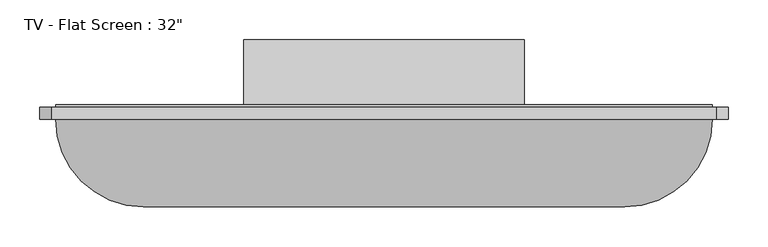
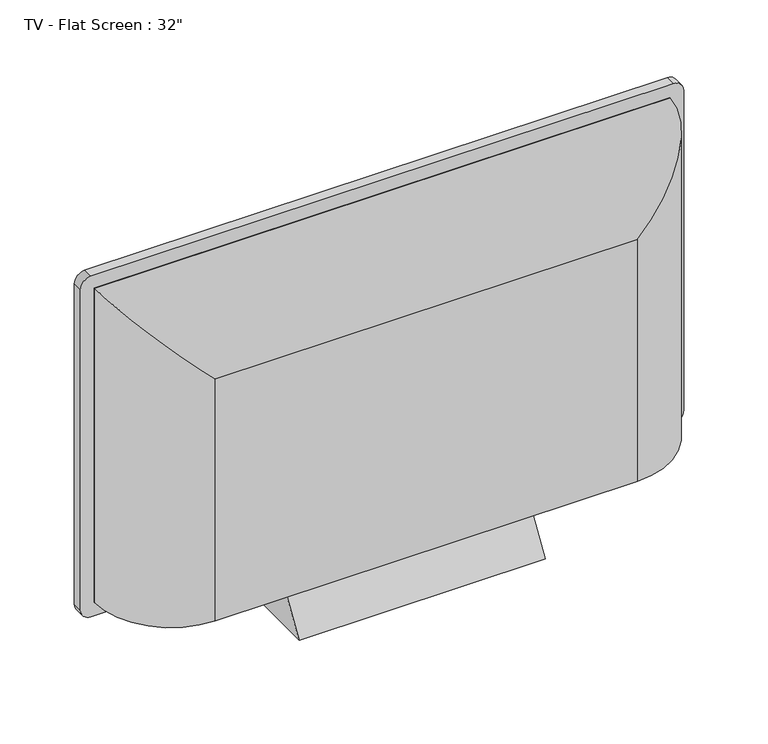
"""IFC4 building model written with IfcOpenShell, lengths in millimetres: furniture geometry."""

from ifc_helpers import new_model, si_unit, point, frame, frame_2d, origin, place, context, project, spatial, polyline, circle_curve, ellipse_curve, trimmed, segment, composite_curve, outline, extrude, faceted_brep, source, transform, mapped, element, save
from ifc_brep_helpers import plane_surface, cylinder_surface, advanced_brep


def furniture_f557e78a(model_context):
    return source(origin(), model_context, "Body", "SolidModel", [
        extrude(outline(polyline([(51.4613764, 80.0), (51.4613764, 20.0), (151.4613764, 10.0), (151.4613764, 0.0), (-48.5386236, 0.0), (1.4613764, 80.0), (51.4613764, 80.0)])), frame((-180.4346678, 0.0, 0.0), z_axis=(1.0, 0.0, 0.0), x_axis=(0.0, 1.0, 0.0)), (0.0, 0.0, 1.0), 352.9803073),
        faceted_brep([(409.0357931, 69.4613764, 557.1392838), (409.0357931, 69.4613764, 80.0), (-416.9248214, 69.4613764, 80.0), (-416.9248214, 69.4613764, 557.1392838), (-356.9248214, 69.4613764, 517.1392838), (-356.9248214, 69.4613764, 120.0), (349.0357931, 69.4613764, 120.0), (349.0357931, 69.4613764, 517.1392838), (409.0357931, 51.4613764, 557.1392838), (-416.9248214, 51.4613764, 557.1392838), (-416.9248214, 51.4613764, 80.0), (409.0357931, 51.4613764, 80.0), (-356.9248214, 66.4613764, 517.1392838), (349.0357931, 66.4613764, 517.1392838), (349.0357931, 66.4613764, 120.0), (-356.9248214, 66.4613764, 120.0)], [[[0, 1, 2, 3], [4, 5, 6, 7]], [[8, 9, 10, 11]], [[3, 9, 8, 0]], [[2, 10, 9, 3]], [[1, 11, 10, 2]], [[0, 8, 11, 1]], [[12, 13, 14, 15]], [[12, 4, 7, 13]], [[13, 7, 6, 14]], [[14, 6, 5, 15]], [[15, 5, 4, 12]]]),
        extrude(outline(composite_curve([segment(polyline([(577.1392838, 414.0357931), (577.1392838, -421.9248214)]), True, "CONTINUOUS"), segment(trimmed(circle_curve(frame_2d((562.1392838, -421.9248214)), 15.0), [point((577.1392838, -421.9248214))], [point((562.1392838, -436.9248214))], False, "CARTESIAN"), True, "CONTINUOUS"), segment(polyline([(562.1392838, -436.9248214), (75.0, -436.9248214)]), True, "CONTINUOUS"), segment(trimmed(circle_curve(frame_2d((75.0, -421.9248214)), 15.0), [point((75.0, -436.9248214))], [point((60.0, -421.9248214))], False, "CARTESIAN"), True, "CONTINUOUS"), segment(polyline([(60.0, -421.9248214), (60.0, 414.0357931)]), True, "CONTINUOUS"), segment(trimmed(circle_curve(frame_2d((75.0, 414.0357931)), 15.0), [point((60.0, 414.0357931))], [point((75.0, 429.0357931))], False, "CARTESIAN"), True, "CONTINUOUS"), segment(polyline([(75.0, 429.0357931), (562.1392838, 429.0357931)]), True, "CONTINUOUS"), segment(trimmed(circle_curve(frame_2d((562.1392838, 414.0357931)), 15.0), [point((562.1392838, 429.0357931))], [point((577.1392838, 414.0357931))], False, "CARTESIAN"), True, "CONTINUOUS")], self_intersect=False), holes=[polyline([(557.1392838, 409.0357931), (80.0, 409.0357931), (80.0, -416.9248214), (557.1392838, -416.9248214), (557.1392838, 409.0357931)])]), frame((0.0, 51.4613764, 0.0), z_axis=(0.0, 1.0, 0.0), x_axis=(0.0, 0.0, 1.0)), (0.0, 0.0, 1.0), 15.0),
        advanced_brep(
        [(-416.9248214, 51.4613764, 80.0), (-416.9248214, 51.4613764, 557.1392838), (409.0357931, 51.4613764, 557.1392838), (409.0357931, 51.4613764, 80.0), (299.0357931, -58.5386236, 80.0), (299.0357931, -58.5386236, 447.1392838), (-306.9248214, -58.5386236, 447.1392838), (-306.9248214, -58.5386236, 80.0)],
        [
            (0, 1),
            (1, 2),
            (2, 3),
            (3, 0),
            (4, 5),
            (5, 6),
            (6, 7),
            (7, 4),
            (3, 4, circle_curve(frame((299.0357931, 51.4613764, 80.0), z_axis=(0.0, 0.0, -1.0), x_axis=(1.0, 0.0, 0.0)), 110.0)),
            (7, 0, circle_curve(frame((-306.9248214, 51.4613764, 80.0), z_axis=(0.0, 0.0, -1.0), x_axis=(-1.0, 0.0, 0.0)), 110.0)),
            (2, 5, ellipse_curve(frame((299.0357931, 51.4613764, 447.1392838), z_axis=(0.7071067811865475, 0.0, -0.7071067811865475), x_axis=(0.7071067811865474, 0.0, 0.7071067811865476)), 155.5634919, 110.0)),
            (1, 6, ellipse_curve(frame((-306.9248214, 51.4613764, 447.1392838), z_axis=(0.7071067811865475, 0.0, 0.7071067811865475), x_axis=(-0.7071067811865476, 0.0, 0.7071067811865474)), 155.5634919, 110.0)),
        ],
        [
            plane_surface(frame((-416.9248214, 51.4613764, 557.1392838), z_axis=(0.0, 1.0, 0.0), x_axis=(-1.0, 0.0, 0.0))),
            plane_surface(frame((-416.9248214, -58.5386236, 557.1392838), z_axis=(0.0, -1.0, 0.0), x_axis=(1.0, 0.0, 0.0))),
            plane_surface(frame((-416.9248214, 51.4613764, 80.0), z_axis=(0.0, 0.0, -1.0), x_axis=(0.0, -1.0, 0.0))),
            cylinder_surface(frame((299.0357931, 51.4613764, 80.0), z_axis=(0.0, 0.0, 1.0), x_axis=(1.0, 0.0, 0.0)), 110.0),
            cylinder_surface(frame((409.0357931, 51.4613764, 447.1392838), z_axis=(-1.0, 0.0, 0.0), x_axis=(0.0, 0.0, 1.0)), 110.0),
            cylinder_surface(frame((-306.9248214, 51.4613764, 557.1392838), z_axis=(0.0, 0.0, -1.0), x_axis=(-1.0, 0.0, 0.0)), 110.0),
        ],
        [
            (0, [[1, 2, 3, 4]]),
            (1, [[5, 6, 7, 8]]),
            (2, [[9, -8, 10, -4]]),
            (3, [[-5, -9, -3, 11]]),
            (4, [[-2, 12, -6, -11]]),
            (5, [[-1, -10, -7, -12]]),
        ],
    ),
    ])


if __name__ == "__main__":
    model = new_model("IFC4")
    model_context = context("Model", 3, world=origin())
    ifc_project = project(units=[si_unit("LENGTHUNIT", "METRE", prefix="MILLI")], contexts=[model_context])
    site = spatial("IfcSite", under=ifc_project)
    building = spatial("IfcBuilding", under=site)
    placement = place(None, origin())
    furniture_shape = furniture_f557e78a(model_context)
    element("IfcFurniture", 1, ObjectType="TV - Flat Screen : 32\"", at=placement, inside=building, context=model_context, shape_type="MappedRepresentation", body=[
        mapped(furniture_shape, transform((0.0, 0.0, 0.0), x_axis=(1.0, 0.0, 0.0), y_axis=(0.0, 1.0, 0.0), z_axis=(0.0, 0.0, 1.0))),
    ])
    save(model, "model.ifc")

# Revit data of these elements
# Type "TV - Flat Screen : 32\""
#   SinAng = 0' - 0.0193"
#   L = 2' - 3.79372"
#   H = 1' - 3.6354"
#   Thickness = 0' - 4.33071"
#   Diagonal = 2' - 7.88976"
#   CosAng = 0' - 0.03431"
#   Stand [instance default] = yes
#   Default Elevation = 0
# Element 1 (IfcFurniture, "TV - Flat Screen : 32\"")
#   Materials on its faces: "TV - Black", "TV - Glass", "TV - Screen"
# Materials
#   "TV - Black": colour RGB 49 49 49, transparency 0
#   "TV - Glass": colour RGB 157 157 157, transparency 0.9
#   "TV - Screen": colour RGB 0 0 0, transparency 0
